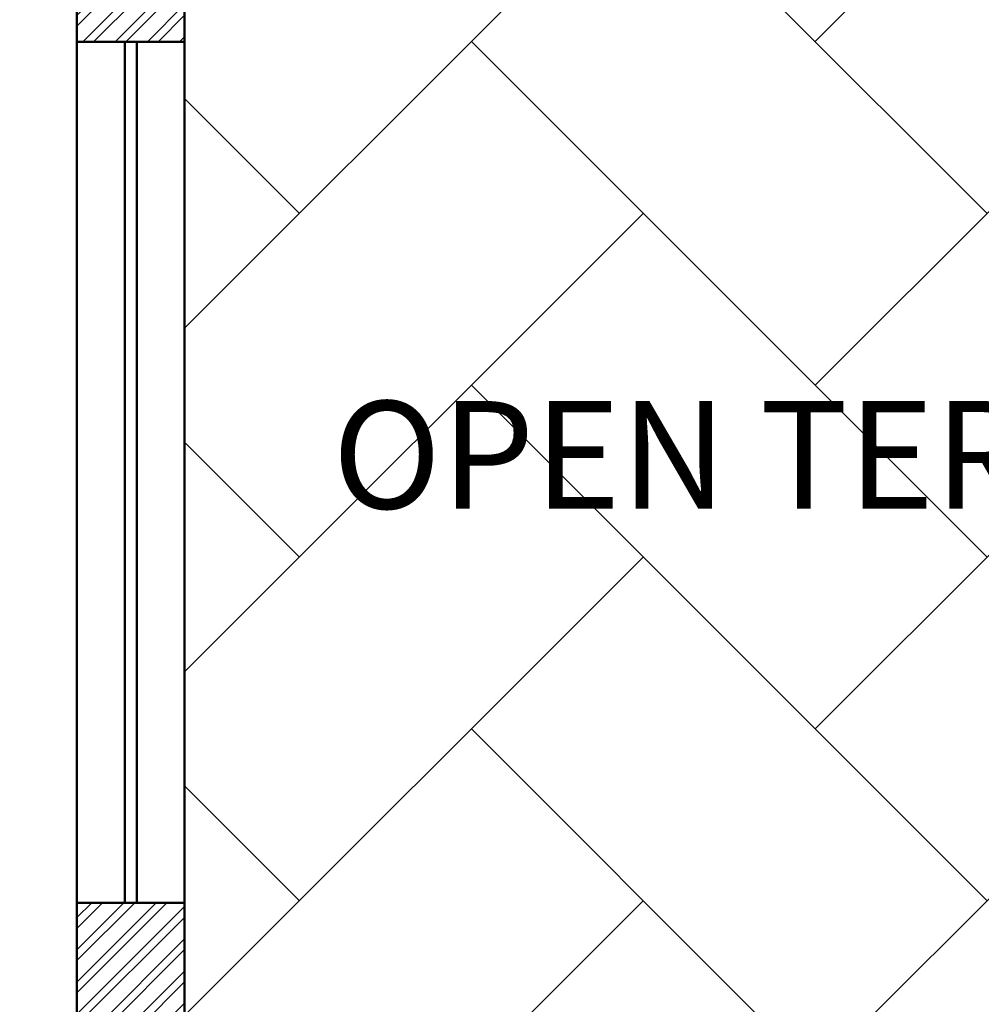
# Model space of a CAD drawing. Units: inches. Extents: x 3590 to 5167, y 65 to 1917.
# Tile 58 of 100: x 4919 to 5000, y 1558 to 1640. Entities that reach past the tile are written whole.
import ezdxf

# ---------------------------------------------------------------- set-up
doc = ezdxf.new("R2010")
doc.units = ezdxf.units.IN
for name, color, linetype, lineweight in [('A-AREA-IDEN', 7, 'Continuous', 18), ('A-FLOR-PATT', 8, 'Continuous', 13), ('A-WALL', 7, 'Continuous', 50), ('A-WALL-PATT', 251, 'Continuous', 13)]:
    doc.layers.add(name, color=color, linetype=linetype, lineweight=lineweight)
doc.styles.get("Standard").update_dxf_attribs({"font": 'arial.ttf'})

msp = doc.modelspace()

# ---------------------------------------------------------------- hatches: boundary and pattern name
at = {"layer": 'A-FLOR-PATT', "transparency": 33554687}
h = msp.add_hatch(dxfattribs=at)
h.set_pattern_fill('AR-HBONE', color=256, scale=0.2)
h.set_pattern_definition([(45, (-588.972, 0), (0, 28.73682), [60.96, -20.32]), (135, (-574.604, 14.368), (3e-15, 28.73682), [60.96, -20.32])])
h.paths.add_polyline_path([(5071.274, 1796.999), (4933.274, 1796.999), (4933.274, 1753.999), (4962.774, 1753.999, -0.414214), (4928.774, 1719.999), (4933.274, 1718.999), (4933.274, 1334.999), (5071.274, 1334.999)])
h.paths.add_polyline_path([(4951.78, 1521.077), (4951.715, 1521.04), (4951.563, 1520.895)], flags=16)
h.paths.add_polyline_path([(4952.267, 1521.376), (4952.198, 1521.371), (4952.198, 1521.356)], flags=0)
h.paths.add_polyline_path([(4967.051, 1529.728), (4965.231, 1528.694), (4963.411, 1527.714), (4961.756, 1526.851), (4963.589, 1527.449), (4964.036, 1527.478), (4962.975, 1527.249), (4961.76, 1526.852), (4959.792, 1525.834), (4958.005, 1524.895), (4956.24, 1523.93), (4954.504, 1522.919), (4954.129, 1522.682), (4953.361, 1521.997), (4953.366, 1521.998), (4953.605, 1522.064), (4955.106, 1522.761), (4956.921, 1523.434), (4958.678, 1523.915), (4960.358, 1524.2), (4961.945, 1524.286), (4964.171, 1524.108), (4965.958, 1523.309), (4963.863, 1522.976), (4965.187, 1522.499), (4963.366, 1522.497), (4961.545, 1522.487), (4959.764, 1522.461), (4958.304, 1522.419), (4957.974, 1522.388), (4956.307, 1522.232), (4954.718, 1522.071), (4953.251, 1521.899), (4953.525, 1521.623), (4954.331, 1521.379), (4956.243, 1521.23), (4958.039, 1520.93), (4959.684, 1520.483), (4961.16, 1519.896), (4963.107, 1518.8), (4964.393, 1517.325), (4962.973, 1517.726), (4964.558, 1516.661), (4965.407, 1515.708), (4963.507, 1516.322), (4961.68, 1517.005), (4959.935, 1517.745), (4958.282, 1518.528), (4956.732, 1519.343), (4955.295, 1520.175), (4954.672, 1520.572), (4954.513, 1520.627), (4955.658, 1519.318), (4956.703, 1517.982), (4957.644, 1516.647), (4958.485, 1515.334), (4959.55, 1513.524), (4960.438, 1511.769), (4958.841, 1513.62), (4957.452, 1515.325), (4955.819, 1517.459), (4956.665, 1515.448), (4957.111, 1513.923), (4957.447, 1511.714), (4957.076, 1509.793), (4956.538, 1511.11), (4955.992, 1512.569), (4955.444, 1514.125), (4954.898, 1515.735), (4954.357, 1517.356), (4953.824, 1518.943), (4953.305, 1520.452), (4953.065, 1521.116), (4952.971, 1521.146), (4952.949, 1521.086), (4952.73, 1520.199), (4953.37, 1518.024), (4953.757, 1516.373), (4954.051, 1514.765), (4954.264, 1513.221), (4954.471, 1511.131), (4954.497, 1510.402), (4954.409, 1511.76), (4954.264, 1513.221), (4954.051, 1514.765), (4953.757, 1516.373), (4953.37, 1518.024), (4952.877, 1519.698), (4952.716, 1520.141), (4952.533, 1519.059), (4952.374, 1517.789), (4952.219, 1516.312), (4952.046, 1514.6), (4951.833, 1512.626), (4951.557, 1510.363), (4951.203, 1512.168), (4950.852, 1514.339), (4950.985, 1516.376), (4951.66, 1518.286), (4952.593, 1520.481), (4952.357, 1521.13), (4951.855, 1520.328), (4950.839, 1518.908), (4949.777, 1517.587), (4948.916, 1516.617), (4948.111, 1515.256), (4947.089, 1513.554), (4945.889, 1511.615), (4946.326, 1513.402), (4946.562, 1514.249), (4945.528, 1513.327), (4944.581, 1512.531), (4946.018, 1514.508), (4947.204, 1516.048), (4947.893, 1517.313), (4949.307, 1518.764), (4950.414, 1519.767), (4950.451, 1519.806), (4952.267, 1521.376), (4951.645, 1521.493), (4950.404, 1521.18), (4948.044, 1520.359), (4946.119, 1519.452), (4944.572, 1518.475), (4943.35, 1517.443), (4941.997, 1515.92), (4941.661, 1515.275), (4942.813, 1516.99), (4944.572, 1518.475), (4946.119, 1519.452), (4948.044, 1520.359), (4950.404, 1521.18), (4951.645, 1521.493), (4949.647, 1521.868), (4948.6, 1521.756), (4947.126, 1521.57), (4945.42, 1521.348), (4943.45, 1521.105), (4941.183, 1520.856), (4942.86, 1521.613), (4943.873, 1522.03), (4942.952, 1521.909), (4941.41, 1521.485), (4939.543, 1520.67), (4938.968, 1520.226), (4940.733, 1521.299), (4942.952, 1521.909), (4943.702, 1522.008), (4945.894, 1522.7), (4947.565, 1522.714), (4948.921, 1522.566), (4951.131, 1522.183), (4950.971, 1522.297), (4948.129, 1523.006), (4946.035, 1523.707), (4944.232, 1524.521), (4942.707, 1525.461), (4941.444, 1526.537), (4940.43, 1527.761), (4939.649, 1529.143), (4941.421, 1528.122), (4943.147, 1527.132), (4944.841, 1526.175), (4946.514, 1525.25), (4948.179, 1524.359), (4948.365, 1524.263), (4946.475, 1526.045), (4945.181, 1527.54), (4944.19, 1529.033), (4943.496, 1530.54), (4943.278, 1531.36), (4942.498, 1531.919), (4943.114, 1531.762), (4942.959, 1533.659), (4944.14, 1531.989), (4944.612, 1531.323), (4946.202, 1530.463), (4947.486, 1529.509), (4948.79, 1528.226), (4950.368, 1526.237), (4949.485, 1528.155), (4948.851, 1530.123), (4948.491, 1532.041), (4948.381, 1533.918), (4948.501, 1535.76), (4948.827, 1537.573), (4949.418, 1535.565), (4949.957, 1533.569), (4950.464, 1531.586), (4950.961, 1529.617), (4951.391, 1527.954), (4951.724, 1530.687), (4952.201, 1532.58), (4952.889, 1534.33), (4953.77, 1535.951), (4954.827, 1537.46), (4954.521, 1535.39), (4954.273, 1533.937), (4955.58, 1535.663), (4956.748, 1536.739), (4956.159, 1534.78), (4955.589, 1532.873), (4955.043, 1531.006), (4954.525, 1529.166), (4954.038, 1527.341), (4953.638, 1525.733), (4953.611, 1525.586), (4953.398, 1524.166), (4953.382, 1524.009), (4954.07, 1525.476), (4954.912, 1527.022), (4956.136, 1528.894), (4957.847, 1530.577), (4959.376, 1531.54), (4958.256, 1530.104), (4957.143, 1528.663), (4956.066, 1527.243), (4955.056, 1525.871), (4954.141, 1524.571), (4953.352, 1523.372), (4953.311, 1523.303), (4953.273, 1522.925), (4953.261, 1522.382), (4954.103, 1523.373), (4954.63, 1524.284), (4955.961, 1526.358), (4957.23, 1528.13), (4958.421, 1529.609), (4960.037, 1531.368), (4961.374, 1532.375), (4962.101, 1532.77), (4961.07, 1531.061), (4959.987, 1529.438), (4958.869, 1527.908), (4958.15, 1527.007), (4959.803, 1528.003), (4961.589, 1528.793), (4963.391, 1529.328), (4965.211, 1529.632)], flags=16)
h.paths.add_polyline_path([(4962.944, 1523.182), (4961.107, 1523.422), (4960.392, 1523.362), (4962.35, 1523.331)], flags=0)
h.paths.add_polyline_path([(5049.541, 1584.551), (5049.476, 1584.515), (5049.325, 1584.37)], flags=16)
h.paths.add_polyline_path([(5050.028, 1584.851), (5049.959, 1584.845), (5049.959, 1584.83)], flags=0)
h.paths.add_polyline_path([(5042.333, 1581.949), (5043.88, 1582.926), (5045.806, 1583.833), (5048.165, 1584.654), (5049.406, 1584.967), (5047.408, 1585.342), (5046.361, 1585.231), (5044.888, 1585.044), (5043.181, 1584.822), (5041.211, 1584.579), (5038.944, 1584.33), (5040.622, 1585.087), (5041.634, 1585.504), (5040.713, 1585.383), (5039.171, 1584.959), (5037.304, 1584.144), (5036.729, 1583.7), (5038.494, 1584.773), (5040.713, 1585.383), (5041.463, 1585.482), (5043.655, 1586.174), (5045.326, 1586.188), (5046.682, 1586.04), (5048.893, 1585.657), (5048.732, 1585.771), (5045.891, 1586.48), (5043.796, 1587.181), (5041.994, 1587.996), (5040.468, 1588.935), (5039.205, 1590.011), (5038.191, 1591.235), (5037.41, 1592.617), (5039.182, 1591.596), (5040.909, 1590.607), (5042.602, 1589.649), (5044.275, 1588.724), (5045.94, 1587.833), (5046.126, 1587.738), (5044.237, 1589.519), (5042.942, 1591.015), (5041.952, 1592.508), (5041.257, 1594.014), (5041.039, 1594.834), (5040.26, 1595.393), (5040.875, 1595.237), (5040.721, 1597.133), (5041.901, 1595.463), (5042.373, 1594.798), (5043.963, 1593.938), (5045.247, 1592.983), (5046.552, 1591.701), (5048.129, 1589.712), (5047.247, 1591.63), (5046.613, 1593.597), (5046.252, 1595.515), (5046.142, 1597.392), (5046.262, 1599.234), (5046.588, 1601.047), (5047.179, 1599.039), (5047.718, 1597.043), (5048.225, 1595.06), (5048.722, 1593.091), (5049.152, 1591.429), (5049.485, 1594.161), (5049.962, 1596.054), (5050.65, 1597.804), (5051.532, 1599.425), (5052.589, 1600.934), (5052.283, 1598.864), (5052.034, 1597.411), (5053.341, 1599.137), (5054.509, 1600.213), (5053.92, 1598.254), (5053.35, 1596.348), (5052.805, 1594.48), (5052.286, 1592.64), (5051.799, 1590.815), (5051.4, 1589.207), (5051.373, 1589.06), (5051.159, 1587.64), (5051.143, 1587.483), (5051.831, 1588.95), (5052.673, 1590.496), (5053.898, 1592.368), (5055.608, 1594.051), (5057.137, 1595.014), (5056.017, 1593.578), (5054.904, 1592.137), (5053.828, 1590.717), (5052.817, 1589.345), (5051.902, 1588.046), (5051.113, 1586.846), (5051.072, 1586.777), (5051.034, 1586.399), (5051.022, 1585.856), (5051.864, 1586.847), (5052.391, 1587.758), (5053.723, 1589.832), (5054.991, 1591.604), (5056.182, 1593.083), (5057.798, 1594.842), (5059.135, 1595.849), (5059.863, 1596.244), (5058.831, 1594.535), (5057.749, 1592.912), (5056.63, 1591.382), (5055.912, 1590.482), (5057.564, 1591.477), (5059.35, 1592.267), (5061.152, 1592.802), (5062.972, 1593.106), (5064.812, 1593.203), (5062.992, 1592.169), (5061.172, 1591.188), (5059.518, 1590.325), (5061.35, 1590.924), (5061.797, 1590.952), (5060.737, 1590.723), (5059.521, 1590.326), (5057.553, 1589.308), (5055.766, 1588.369), (5054.002, 1587.404), (5052.265, 1586.393), (5051.891, 1586.156), (5051.122, 1585.471), (5051.127, 1585.472), (5051.366, 1585.538), (5052.867, 1586.235), (5054.682, 1586.908), (5056.439, 1587.389), (5058.12, 1587.675), (5059.706, 1587.76), (5061.933, 1587.583), (5063.719, 1586.783), (5061.624, 1586.45), (5062.949, 1585.973), (5061.127, 1585.971), (5059.307, 1585.961), (5057.525, 1585.935), (5056.065, 1585.893), (5055.735, 1585.862), (5054.068, 1585.707), (5052.479, 1585.546), (5051.012, 1585.373), (5051.286, 1585.097), (5052.092, 1584.853), (5054.004, 1584.704), (5055.8, 1584.404), (5057.446, 1583.958), (5058.921, 1583.37), (5060.868, 1582.274), (5062.154, 1580.799), (5060.734, 1581.2), (5062.32, 1580.135), (5063.168, 1579.182), (5061.269, 1579.796), (5059.441, 1580.479), (5057.696, 1581.219), (5056.043, 1582.003), (5054.493, 1582.817), (5053.057, 1583.649), (5052.433, 1584.047), (5052.274, 1584.101), (5053.42, 1582.793), (5054.464, 1581.457), (5055.405, 1580.121), (5056.247, 1578.809), (5057.311, 1576.998), (5058.199, 1575.244), (5056.602, 1577.094), (5055.213, 1578.799), (5053.58, 1580.933), (5054.427, 1578.922), (5054.872, 1577.397), (5055.208, 1575.189), (5054.838, 1573.267), (5054.299, 1574.584), (5053.754, 1576.043), (5053.206, 1577.599), (5052.659, 1579.209), (5052.118, 1580.83), (5051.585, 1582.417), (5051.066, 1583.927), (5050.826, 1584.59), (5050.733, 1584.62), (5050.711, 1584.561), (5050.491, 1583.673), (5051.131, 1581.498), (5051.518, 1579.847), (5051.813, 1578.24), (5052.026, 1576.695), (5052.233, 1574.605), (5052.258, 1573.876), (5052.17, 1575.234), (5052.026, 1576.695), (5051.813, 1578.24), (5051.518, 1579.847), (5051.131, 1581.498), (5050.638, 1583.172), (5050.477, 1583.615), (5050.294, 1582.533), (5050.136, 1581.263), (5049.981, 1579.786), (5049.807, 1578.074), (5049.594, 1576.1), (5049.318, 1573.837), (5048.965, 1575.642), (5048.613, 1577.813), (5048.747, 1579.85), (5049.421, 1581.76), (5050.354, 1583.955), (5050.118, 1584.604), (5049.616, 1583.802), (5048.6, 1582.382), (5047.538, 1581.061), (5046.677, 1580.091), (5045.872, 1578.73), (5044.85, 1577.028), (5043.651, 1575.089), (5044.087, 1576.877), (5044.324, 1577.723), (5043.289, 1576.801), (5042.342, 1576.005), (5043.779, 1577.982), (5044.966, 1579.522), (5045.655, 1580.787), (5047.068, 1582.239), (5048.175, 1583.241), (5048.213, 1583.28), (5050.028, 1584.851), (5049.406, 1584.967), (5048.165, 1584.654), (5045.806, 1583.833), (5043.88, 1582.926), (5042.333, 1581.949), (5041.111, 1580.917), (5039.758, 1579.394), (5039.423, 1578.749), (5040.575, 1580.464)], flags=16)
h.paths.add_polyline_path([(4954.799, 1533.12), (4954.262, 1532.079), (4953.831, 1530.935), (4953.505, 1529.636), (4953.283, 1528.133), (4953.167, 1526.376), (4953.156, 1524.315), (4953.277, 1521.236), (4952.802, 1521.842), (4951.557, 1521.998), (4950.976, 1521.961), (4952.661, 1521.941), (4952.802, 1521.842), (4953.152, 1523.593), (4953.167, 1526.376), (4953.283, 1528.133), (4953.609, 1530.346), (4954.456, 1532.592)], flags=0)
h.paths.add_polyline_path([(5050.563, 1585.316), (5049.318, 1585.472), (5048.737, 1585.435), (5050.422, 1585.415), (5050.563, 1585.316), (5050.914, 1587.067), (5050.928, 1589.851), (5051.045, 1591.607), (5051.371, 1593.82), (5052.217, 1596.066), (5052.56, 1596.594), (5052.024, 1595.554), (5051.592, 1594.409), (5051.266, 1593.11), (5051.045, 1591.607), (5050.928, 1589.851), (5050.918, 1587.789), (5051.038, 1584.71)], flags=0)
h.paths.add_polyline_path([(5058.153, 1586.836), (5060.111, 1586.805), (5060.705, 1586.656), (5058.868, 1586.896)], flags=0)
h.paths.add_polyline_path([(5049.541, 1430.936), (5049.476, 1430.9), (5049.325, 1430.755)], flags=16)
h.paths.add_polyline_path([(5050.028, 1431.236), (5049.959, 1431.231), (5049.959, 1431.215)], flags=0)
h.paths.add_polyline_path([(5046.588, 1447.432), (5047.179, 1445.425), (5047.718, 1443.429), (5048.225, 1441.446), (5048.722, 1439.476), (5049.152, 1437.814), (5049.485, 1440.546), (5049.962, 1442.439), (5050.65, 1444.189), (5051.532, 1445.811), (5052.589, 1447.319), (5052.283, 1445.249), (5052.034, 1443.796), (5053.341, 1445.522), (5054.509, 1446.598), (5053.92, 1444.64), (5053.35, 1442.733), (5052.805, 1440.865), (5052.286, 1439.025), (5051.799, 1437.201), (5051.4, 1435.592), (5051.373, 1435.445), (5051.159, 1434.025), (5051.143, 1433.868), (5051.831, 1435.335), (5052.673, 1436.881), (5053.898, 1438.753), (5055.608, 1440.436), (5057.137, 1441.4), (5056.017, 1439.963), (5054.904, 1438.522), (5053.828, 1437.102), (5052.817, 1435.73), (5051.902, 1434.431), (5051.113, 1433.231), (5051.072, 1433.162), (5051.034, 1432.784), (5051.022, 1432.242), (5051.864, 1433.232), (5052.391, 1434.143), (5053.723, 1436.217), (5054.991, 1437.989), (5056.182, 1439.468), (5057.798, 1441.227), (5059.135, 1442.235), (5059.863, 1442.629), (5058.831, 1440.921), (5057.749, 1439.298), (5056.63, 1437.767), (5055.912, 1436.867), (5057.564, 1437.863), (5059.35, 1438.652), (5061.152, 1439.187), (5062.972, 1439.491), (5064.812, 1439.588), (5062.992, 1438.554), (5061.172, 1437.573), (5059.518, 1436.71), (5061.35, 1437.309), (5061.797, 1437.337), (5060.737, 1437.108), (5059.521, 1436.711), (5057.553, 1435.693), (5055.766, 1434.754), (5054.002, 1433.789), (5052.265, 1432.778), (5051.891, 1432.541), (5051.122, 1431.856), (5051.127, 1431.857), (5051.366, 1431.923), (5052.867, 1432.62), (5054.682, 1433.293), (5056.439, 1433.775), (5058.12, 1434.06), (5059.706, 1434.145), (5061.933, 1433.968), (5063.719, 1433.168), (5061.624, 1432.835), (5062.949, 1432.358), (5061.127, 1432.357), (5059.307, 1432.346), (5057.525, 1432.32), (5056.065, 1432.278), (5055.735, 1432.248), (5054.068, 1432.092), (5052.479, 1431.931), (5051.012, 1431.759), (5051.286, 1431.482), (5052.092, 1431.238), (5054.004, 1431.089), (5055.8, 1430.789), (5057.446, 1430.343), (5058.921, 1429.755), (5060.868, 1428.66), (5062.154, 1427.185), (5060.734, 1427.585), (5062.32, 1426.52), (5063.168, 1425.567), (5061.269, 1426.181), (5059.441, 1426.865), (5057.696, 1427.604), (5056.043, 1428.388), (5054.493, 1429.202), (5053.057, 1430.034), (5052.433, 1430.432), (5052.274, 1430.487), (5053.42, 1429.178), (5054.464, 1427.842), (5055.405, 1426.506), (5056.247, 1425.194), (5057.311, 1423.383), (5058.199, 1421.629), (5056.602, 1423.479), (5055.213, 1425.184), (5053.58, 1427.318), (5054.427, 1425.307), (5054.872, 1423.782), (5055.208, 1421.574), (5054.838, 1419.652), (5054.299, 1420.97), (5053.754, 1422.428), (5053.206, 1423.984), (5052.659, 1425.595), (5052.118, 1427.215), (5051.585, 1428.802), (5051.066, 1430.312), (5050.826, 1430.975), (5050.733, 1431.005), (5050.711, 1430.946), (5050.491, 1430.058), (5051.131, 1427.883), (5051.518, 1426.232), (5051.813, 1424.625), (5052.026, 1423.081), (5052.233, 1420.991), (5052.258, 1420.261), (5052.17, 1421.619), (5052.026, 1423.081), (5051.813, 1424.625), (5051.518, 1426.232), (5051.131, 1427.883), (5050.638, 1429.558), (5050.477, 1430.001), (5050.294, 1428.918), (5050.136, 1427.648), (5049.981, 1426.171), (5049.807, 1424.459), (5049.594, 1422.485), (5049.318, 1420.222), (5048.965, 1422.028), (5048.613, 1424.199), (5048.747, 1426.235), (5049.421, 1428.146), (5050.354, 1430.34), (5050.118, 1430.989), (5049.616, 1430.187), (5048.6, 1428.768), (5047.538, 1427.446), (5046.677, 1426.477), (5045.872, 1425.116), (5044.85, 1423.413), (5043.651, 1421.474), (5044.087, 1423.262), (5044.324, 1424.109), (5043.289, 1423.186), (5042.342, 1422.391), (5043.779, 1424.368), (5044.966, 1425.907), (5045.655, 1427.173), (5047.068, 1428.624), (5048.175, 1429.627), (5048.213, 1429.666), (5050.028, 1431.236), (5049.406, 1431.353), (5048.165, 1431.039), (5045.806, 1430.218), (5043.88, 1429.311), (5042.333, 1428.334), (5041.111, 1427.302), (5039.758, 1425.779), (5039.423, 1425.134), (5040.575, 1426.849), (5042.333, 1428.334), (5043.88, 1429.311), (5045.806, 1430.218), (5048.165, 1431.039), (5049.406, 1431.353), (5047.408, 1431.727), (5046.361, 1431.616), (5044.888, 1431.429), (5043.181, 1431.207), (5041.211, 1430.964), (5038.944, 1430.715), (5040.622, 1431.472), (5041.634, 1431.89), (5040.713, 1431.769), (5039.171, 1431.345), (5037.304, 1430.53), (5036.729, 1430.085), (5038.494, 1431.158), (5040.713, 1431.769), (5041.463, 1431.867), (5043.655, 1432.559), (5045.326, 1432.573), (5046.682, 1432.425), (5048.893, 1432.042), (5048.732, 1432.156), (5045.891, 1432.865), (5043.796, 1433.566), (5041.994, 1434.381), (5040.468, 1435.321), (5039.205, 1436.396), (5038.191, 1437.62), (5037.41, 1439.002), (5039.182, 1437.982), (5040.909, 1436.992), (5042.602, 1436.034), (5044.275, 1435.109), (5045.94, 1434.218), (5046.126, 1434.123), (5044.237, 1435.904), (5042.942, 1437.4), (5041.952, 1438.893), (5041.257, 1440.399), (5041.039, 1441.219), (5040.26, 1441.778), (5040.875, 1441.622), (5040.721, 1443.518), (5041.901, 1441.848), (5042.373, 1441.183), (5043.963, 1440.323), (5045.247, 1439.369), (5046.552, 1438.086), (5048.129, 1436.097), (5047.247, 1438.015), (5046.613, 1439.982), (5046.252, 1441.901), (5046.142, 1443.778), (5046.262, 1445.619)], flags=16)
h.paths.add_polyline_path([(5052.382, 1444.255), (5051.623, 1442.78), (5052.024, 1441.939), (5052.56, 1442.98)], flags=0)
h.paths.add_polyline_path([(5050.563, 1431.701), (5049.318, 1431.857), (5048.737, 1431.821), (5050.422, 1431.8)], flags=0)
h.paths.add_polyline_path([(5058.153, 1433.221), (5060.111, 1433.19), (5060.705, 1433.041), (5058.868, 1433.281)], flags=0)
h.paths.add_polyline_path([(5049.541, 1352.285), (5049.476, 1352.249), (5049.325, 1352.104)], flags=16)
h.paths.add_polyline_path([(5050.028, 1352.585), (5049.959, 1352.58), (5049.959, 1352.564)], flags=0)
h.paths.add_polyline_path([(5046.588, 1368.781), (5047.179, 1366.774), (5047.718, 1364.778), (5048.225, 1362.795), (5048.722, 1360.825), (5049.152, 1359.163), (5049.485, 1361.896), (5049.962, 1363.789), (5050.65, 1365.538), (5051.532, 1367.16), (5052.589, 1368.669), (5052.283, 1366.598), (5052.034, 1365.145), (5053.341, 1366.871), (5054.509, 1367.947), (5053.92, 1365.989), (5053.35, 1364.082), (5052.805, 1362.214), (5052.286, 1360.374), (5051.799, 1358.55), (5051.4, 1356.942), (5051.373, 1356.794), (5051.159, 1355.374), (5051.143, 1355.218), (5051.831, 1356.684), (5052.673, 1358.23), (5053.898, 1360.102), (5055.608, 1361.786), (5057.137, 1362.749), (5056.017, 1361.313), (5054.904, 1359.872), (5053.828, 1358.452), (5052.817, 1357.079), (5051.902, 1355.78), (5051.113, 1354.581), (5051.072, 1354.512), (5051.034, 1354.133), (5051.022, 1353.591), (5051.864, 1354.581), (5052.391, 1355.492), (5053.723, 1357.566), (5054.991, 1359.338), (5056.182, 1360.817), (5057.798, 1362.577), (5059.135, 1363.584), (5059.863, 1363.979), (5058.831, 1362.27), (5057.749, 1360.647), (5056.63, 1359.117), (5055.912, 1358.216), (5057.564, 1359.212), (5059.35, 1360.001), (5061.152, 1360.536), (5062.972, 1360.841), (5064.812, 1360.937), (5062.992, 1359.903), (5061.172, 1358.923), (5059.518, 1358.059), (5061.35, 1358.658), (5061.797, 1358.687), (5060.737, 1358.458), (5059.521, 1358.061), (5057.553, 1357.043), (5055.766, 1356.103), (5054.002, 1355.138), (5052.265, 1354.127), (5051.891, 1353.89), (5051.122, 1353.206), (5051.127, 1353.206), (5051.366, 1353.272), (5052.867, 1353.969), (5054.682, 1354.643), (5056.439, 1355.124), (5058.12, 1355.409), (5059.706, 1355.495), (5061.933, 1355.317), (5063.719, 1354.518), (5061.624, 1354.184), (5062.949, 1353.708), (5061.127, 1353.706), (5059.307, 1353.695), (5057.525, 1353.669), (5056.065, 1353.627), (5055.735, 1353.597), (5054.068, 1353.441), (5052.479, 1353.28), (5051.012, 1353.108), (5051.286, 1352.831), (5052.092, 1352.587), (5054.004, 1352.439), (5055.8, 1352.138), (5057.446, 1351.692), (5058.921, 1351.104), (5060.868, 1350.009), (5062.154, 1348.534), (5060.734, 1348.935), (5062.32, 1347.869), (5063.168, 1346.916), (5061.269, 1347.53), (5059.441, 1348.214), (5057.696, 1348.954), (5056.043, 1349.737), (5054.493, 1350.551), (5053.057, 1351.383), (5052.433, 1351.781), (5052.274, 1351.836), (5053.42, 1350.527), (5054.464, 1349.191), (5055.405, 1347.855), (5056.247, 1346.543), (5057.311, 1344.733), (5058.199, 1342.978), (5056.602, 1344.828), (5055.213, 1346.534), (5053.58, 1348.667), (5054.427, 1346.656), (5054.872, 1345.132), (5055.208, 1342.923), (5054.838, 1341.002), (5054.299, 1342.319), (5053.754, 1343.778), (5053.206, 1345.334), (5052.659, 1346.944), (5052.118, 1348.564), (5051.585, 1350.151), (5051.066, 1351.661), (5050.826, 1352.324), (5050.733, 1352.355), (5050.711, 1352.295), (5050.491, 1351.408), (5051.131, 1349.232), (5051.518, 1347.581), (5051.813, 1345.974), (5052.026, 1344.43), (5052.233, 1342.34), (5052.258, 1341.61), (5052.17, 1342.969), (5052.026, 1344.43), (5051.813, 1345.974), (5051.518, 1347.581), (5051.131, 1349.232), (5050.638, 1350.907), (5050.477, 1351.35), (5050.294, 1350.267), (5050.136, 1348.997), (5049.981, 1347.52), (5049.807, 1345.809), (5049.594, 1343.835), (5049.318, 1341.571), (5048.965, 1343.377), (5048.613, 1345.548), (5048.747, 1347.585), (5049.421, 1349.495), (5050.354, 1351.689), (5050.118, 1352.339), (5049.616, 1351.536), (5048.6, 1350.117), (5047.538, 1348.795), (5046.677, 1347.826), (5045.872, 1346.465), (5044.85, 1344.763), (5043.651, 1342.824), (5044.087, 1344.611), (5044.324, 1345.458), (5043.289, 1344.535), (5042.342, 1343.74), (5043.779, 1345.717), (5044.966, 1347.256), (5045.655, 1348.522), (5047.068, 1349.973), (5048.175, 1350.976), (5048.213, 1351.015), (5050.028, 1352.585), (5049.406, 1352.702), (5048.165, 1352.388), (5045.806, 1351.567), (5043.88, 1350.661), (5042.333, 1349.683), (5041.111, 1348.651), (5039.758, 1347.128), (5039.423, 1346.483), (5040.575, 1348.198), (5042.333, 1349.683), (5043.88, 1350.661), (5045.806, 1351.567), (5048.165, 1352.388), (5049.406, 1352.702), (5047.408, 1353.076), (5046.361, 1352.965), (5044.888, 1352.779), (5043.181, 1352.556), (5041.211, 1352.313), (5038.944, 1352.065), (5040.622, 1352.821), (5041.634, 1353.239), (5040.713, 1353.118), (5039.171, 1352.694), (5037.304, 1351.879), (5036.729, 1351.434), (5038.494, 1352.508), (5040.713, 1353.118), (5041.463, 1353.216), (5043.655, 1353.909), (5045.326, 1353.923), (5046.682, 1353.774), (5048.893, 1353.391), (5048.732, 1353.506), (5045.891, 1354.214), (5043.796, 1354.915), (5041.994, 1355.73), (5040.468, 1356.67), (5039.205, 1357.746), (5038.191, 1358.969), (5037.41, 1360.352), (5039.182, 1359.331), (5040.909, 1358.341), (5042.602, 1357.383), (5044.275, 1356.458), (5045.94, 1355.567), (5046.126, 1355.472), (5044.237, 1357.253), (5042.942, 1358.749), (5041.952, 1360.242), (5041.257, 1361.748), (5041.039, 1362.568), (5040.26, 1363.128), (5040.875, 1362.971), (5040.721, 1364.867), (5041.901, 1363.197), (5042.373, 1362.532), (5043.963, 1361.672), (5045.247, 1360.718), (5046.552, 1359.435), (5048.129, 1357.446), (5047.247, 1359.364), (5046.613, 1361.331), (5046.252, 1363.25), (5046.142, 1365.127), (5046.262, 1366.969)], flags=16)
h.paths.add_polyline_path([(5052.382, 1365.604), (5051.623, 1364.129), (5052.024, 1363.288), (5052.56, 1364.329)], flags=0)
h.paths.add_polyline_path([(4951.78, 1698.041), (4951.715, 1698.005), (4951.563, 1697.859)], flags=16)
h.paths.add_polyline_path([(4952.267, 1698.341), (4952.198, 1698.335), (4952.198, 1698.32)], flags=0)
h.paths.add_polyline_path([(4957.076, 1686.757), (4956.538, 1688.074), (4955.992, 1689.533), (4955.444, 1691.089), (4954.898, 1692.699), (4954.357, 1694.32), (4953.824, 1695.907), (4953.305, 1697.417), (4953.065, 1698.08), (4952.971, 1698.11), (4952.949, 1698.051), (4952.73, 1697.163), (4953.37, 1694.988), (4953.757, 1693.337), (4954.051, 1691.729), (4954.264, 1690.185), (4954.471, 1688.095), (4954.497, 1687.366), (4954.409, 1688.724), (4954.264, 1690.185), (4954.051, 1691.729), (4953.757, 1693.337), (4953.37, 1694.988), (4952.877, 1696.662), (4952.716, 1697.105), (4952.533, 1696.023), (4952.374, 1694.753), (4952.219, 1693.276), (4952.046, 1691.564), (4951.833, 1689.59), (4951.557, 1687.327), (4951.203, 1689.132), (4950.852, 1691.303), (4950.985, 1693.34), (4951.66, 1695.25), (4952.593, 1697.445), (4952.357, 1698.094), (4951.855, 1697.292), (4950.839, 1695.872), (4949.777, 1694.551), (4948.916, 1693.581), (4948.111, 1692.22), (4947.089, 1690.518), (4945.889, 1688.579), (4946.326, 1690.366), (4946.562, 1691.213), (4945.528, 1690.291), (4944.581, 1689.495), (4946.018, 1691.472), (4947.204, 1693.012), (4947.893, 1694.277), (4949.307, 1695.729), (4950.414, 1696.731), (4950.451, 1696.77), (4952.267, 1698.341), (4951.645, 1698.457), (4950.404, 1698.144), (4948.044, 1697.323), (4946.119, 1696.416), (4944.572, 1695.439), (4943.35, 1694.407), (4941.997, 1692.884), (4941.661, 1692.239), (4942.813, 1693.954), (4944.572, 1695.439), (4946.119, 1696.416), (4948.044, 1697.323), (4950.404, 1698.144), (4951.645, 1698.457), (4949.647, 1698.832), (4948.6, 1698.72), (4947.126, 1698.534), (4945.42, 1698.312), (4943.45, 1698.069), (4941.183, 1697.82), (4942.86, 1698.577), (4943.873, 1698.994), (4942.952, 1698.873), (4941.41, 1698.449), (4939.543, 1697.634), (4938.968, 1697.19), (4940.733, 1698.263), (4942.952, 1698.873), (4943.702, 1698.972), (4945.894, 1699.664), (4947.565, 1699.678), (4948.921, 1699.53), (4951.131, 1699.147), (4950.971, 1699.261), (4948.129, 1699.97), (4946.035, 1700.671), (4944.232, 1701.486), (4942.707, 1702.425), (4941.444, 1703.501), (4940.43, 1704.725), (4939.649, 1706.107), (4941.421, 1705.086), (4943.147, 1704.097), (4944.841, 1703.139), (4946.514, 1702.214), (4948.179, 1701.323), (4948.365, 1701.227), (4946.475, 1703.009), (4945.181, 1704.505), (4944.19, 1705.997), (4943.496, 1707.504), (4943.278, 1708.324), (4942.498, 1708.883), (4943.114, 1708.727), (4942.959, 1710.623), (4944.14, 1708.953), (4944.612, 1708.287), (4946.202, 1707.428), (4947.486, 1706.473), (4948.79, 1705.191), (4950.368, 1703.202), (4949.485, 1705.12), (4948.851, 1707.087), (4948.491, 1709.005), (4948.381, 1710.882), (4948.501, 1712.724), (4948.827, 1714.537), (4949.418, 1712.529), (4949.957, 1710.533), (4950.464, 1708.55), (4950.961, 1706.581), (4951.391, 1704.919), (4951.724, 1707.651), (4952.201, 1709.544), (4952.889, 1711.294), (4953.77, 1712.915), (4954.827, 1714.424), (4954.521, 1712.354), (4954.273, 1710.901), (4955.58, 1712.627), (4956.748, 1713.703), (4956.159, 1711.744), (4955.589, 1709.837), (4955.043, 1707.97), (4954.525, 1706.13), (4954.038, 1704.305), (4953.638, 1702.697), (4953.611, 1702.55), (4953.398, 1701.13), (4953.382, 1700.973), (4954.07, 1702.44), (4954.912, 1703.986), (4956.136, 1705.858), (4957.847, 1707.541), (4959.376, 1708.504), (4958.256, 1707.068), (4957.143, 1705.627), (4956.066, 1704.207), (4955.056, 1702.835), (4954.141, 1701.536), (4953.352, 1700.336), (4953.311, 1700.267), (4953.273, 1699.889), (4953.261, 1699.346), (4954.103, 1700.337), (4954.63, 1701.248), (4955.961, 1703.322), (4957.23, 1705.094), (4958.421, 1706.573), (4960.037, 1708.332), (4961.374, 1709.339), (4962.101, 1709.734), (4961.07, 1708.025), (4959.987, 1706.402), (4958.869, 1704.872), (4958.15, 1703.972), (4959.803, 1704.967), (4961.589, 1705.757), (4963.391, 1706.292), (4965.211, 1706.596), (4967.051, 1706.692), (4965.231, 1705.659), (4963.411, 1704.678), (4961.756, 1703.815), (4963.589, 1704.413), (4964.036, 1704.442), (4962.975, 1704.213), (4961.76, 1703.816), (4959.792, 1702.798), (4958.005, 1701.859), (4956.24, 1700.894), (4954.504, 1699.883), (4954.129, 1699.646), (4953.361, 1698.961), (4953.366, 1698.962), (4953.605, 1699.028), (4955.106, 1699.725), (4956.921, 1700.398), (4958.678, 1700.879), (4960.358, 1701.164), (4961.945, 1701.25), (4964.171, 1701.073), (4965.958, 1700.273), (4963.863, 1699.94), (4965.187, 1699.463), (4963.366, 1699.461), (4961.545, 1699.451), (4959.764, 1699.425), (4958.304, 1699.383), (4957.974, 1699.352), (4956.307, 1699.197), (4954.718, 1699.036), (4953.251, 1698.863), (4953.525, 1698.587), (4954.331, 1698.343), (4956.243, 1698.194), (4958.039, 1697.894), (4959.684, 1697.447), (4961.16, 1696.86), (4963.107, 1695.764), (4964.393, 1694.289), (4962.973, 1694.69), (4964.558, 1693.625), (4965.407, 1692.672), (4963.507, 1693.286), (4961.68, 1693.969), (4959.935, 1694.709), (4958.282, 1695.492), (4956.732, 1696.307), (4955.295, 1697.139), (4954.672, 1697.536), (4954.513, 1697.591), (4955.658, 1696.282), (4956.703, 1694.946), (4957.644, 1693.611), (4958.485, 1692.298), (4959.55, 1690.488), (4960.438, 1688.733), (4958.841, 1690.584), (4957.452, 1692.289), (4955.819, 1694.423), (4956.665, 1692.412), (4957.111, 1690.887), (4957.447, 1688.678)], flags=16)
h.paths.add_polyline_path([(5050.563, 1353.05), (5049.318, 1353.207), (5048.737, 1353.17), (5050.422, 1353.15)], flags=0)
h.paths.add_polyline_path([(4951.78, 1351.486), (4951.715, 1351.45), (4951.563, 1351.305)], flags=16)
h.paths.add_polyline_path([(4952.267, 1351.786), (4952.198, 1351.78), (4952.198, 1351.765)], flags=0)
h.paths.add_polyline_path([(4954.827, 1367.869), (4954.521, 1365.799), (4954.273, 1364.346), (4955.58, 1366.072), (4956.748, 1367.148), (4956.159, 1365.19), (4955.589, 1363.283), (4955.043, 1361.415), (4954.525, 1359.575), (4954.038, 1357.751), (4953.638, 1356.142), (4953.611, 1355.995), (4953.398, 1354.575), (4953.382, 1354.418), (4954.07, 1355.885), (4954.912, 1357.431), (4956.136, 1359.303), (4957.847, 1360.986), (4959.376, 1361.95), (4958.256, 1360.513), (4957.143, 1359.072), (4956.066, 1357.652), (4955.056, 1356.28), (4954.141, 1354.981), (4953.352, 1353.781), (4953.311, 1353.712), (4953.273, 1353.334), (4953.261, 1352.792), (4954.103, 1353.782), (4954.63, 1354.693), (4955.961, 1356.767), (4957.23, 1358.539), (4958.421, 1360.018), (4960.037, 1361.777), (4961.374, 1362.785), (4962.101, 1363.179), (4961.07, 1361.471), (4959.987, 1359.848), (4958.869, 1358.317), (4958.15, 1357.417), (4959.803, 1358.413), (4961.589, 1359.202), (4963.391, 1359.737), (4965.211, 1360.041), (4967.051, 1360.138), (4965.231, 1359.104), (4963.411, 1358.123), (4961.756, 1357.26), (4963.589, 1357.859), (4964.036, 1357.887), (4962.975, 1357.658), (4961.76, 1357.261), (4959.792, 1356.243), (4958.005, 1355.304), (4956.24, 1354.339), (4954.504, 1353.328), (4954.129, 1353.091), (4953.361, 1352.406), (4953.366, 1352.407), (4953.605, 1352.473), (4955.106, 1353.17), (4956.921, 1353.843), (4958.678, 1354.325), (4960.358, 1354.61), (4961.945, 1354.695), (4964.171, 1354.518), (4965.958, 1353.718), (4963.863, 1353.385), (4965.187, 1352.908), (4963.366, 1352.907), (4961.545, 1352.896), (4959.764, 1352.87), (4958.304, 1352.828), (4957.974, 1352.798), (4956.307, 1352.642), (4954.718, 1352.481), (4953.251, 1352.309), (4953.525, 1352.032), (4954.331, 1351.788), (4956.243, 1351.639), (4958.039, 1351.339), (4959.684, 1350.893), (4961.16, 1350.305), (4963.107, 1349.21), (4964.393, 1347.735), (4962.973, 1348.135), (4964.558, 1347.07), (4965.407, 1346.117), (4963.507, 1346.731), (4961.68, 1347.414), (4959.935, 1348.154), (4958.282, 1348.938), (4956.732, 1349.752), (4955.295, 1350.584), (4954.672, 1350.982), (4954.513, 1351.036), (4955.658, 1349.728), (4956.703, 1348.392), (4957.644, 1347.056), (4958.485, 1345.744), (4959.55, 1343.933), (4960.438, 1342.179), (4958.841, 1344.029), (4957.452, 1345.734), (4955.819, 1347.868), (4956.665, 1345.857), (4957.111, 1344.332), (4957.447, 1342.124), (4957.076, 1340.202), (4956.538, 1341.52), (4955.992, 1342.978), (4955.444, 1344.534), (4954.898, 1346.145), (4954.357, 1347.765), (4953.824, 1349.352), (4953.305, 1350.862), (4953.065, 1351.525), (4952.971, 1351.555), (4952.949, 1351.496), (4952.73, 1350.608), (4953.37, 1348.433), (4953.757, 1346.782), (4954.051, 1345.175), (4954.264, 1343.631), (4954.471, 1341.541), (4954.497, 1340.811), (4954.409, 1342.169), (4954.264, 1343.631), (4954.051, 1345.175), (4953.757, 1346.782), (4953.37, 1348.433), (4952.877, 1350.108), (4952.716, 1350.551), (4952.533, 1349.468), (4952.374, 1348.198), (4952.219, 1346.721), (4952.046, 1345.009), (4951.833, 1343.035), (4951.557, 1340.772), (4951.203, 1342.578), (4950.852, 1344.749), (4950.985, 1346.785), (4951.66, 1348.696), (4952.593, 1350.89), (4952.357, 1351.539), (4951.855, 1350.737), (4950.839, 1349.318), (4949.777, 1347.996), (4948.916, 1347.027), (4948.111, 1345.665), (4947.089, 1343.963), (4945.889, 1342.024), (4946.326, 1343.812), (4946.562, 1344.659), (4945.528, 1343.736), (4944.581, 1342.941), (4946.018, 1344.918), (4947.204, 1346.457), (4947.893, 1347.723), (4949.307, 1349.174), (4950.414, 1350.177), (4950.451, 1350.216), (4952.267, 1351.786), (4951.645, 1351.903), (4950.404, 1351.589), (4948.044, 1350.768), (4946.119, 1349.861), (4944.572, 1348.884), (4943.35, 1347.852), (4941.997, 1346.329), (4941.661, 1345.684), (4942.813, 1347.399), (4944.572, 1348.884), (4946.119, 1349.861), (4948.044, 1350.768), (4950.404, 1351.589), (4951.645, 1351.903), (4949.647, 1352.277), (4948.6, 1352.166), (4947.126, 1351.979), (4945.42, 1351.757), (4943.45, 1351.514), (4941.183, 1351.265), (4942.86, 1352.022), (4943.873, 1352.44), (4942.952, 1352.319), (4941.41, 1351.895), (4939.543, 1351.08), (4938.968, 1350.635), (4940.733, 1351.708), (4942.952, 1352.319), (4943.702, 1352.417), (4945.894, 1353.109), (4947.565, 1353.123), (4948.921, 1352.975), (4951.131, 1352.592), (4950.971, 1352.706), (4948.129, 1353.415), (4946.035, 1354.116), (4944.232, 1354.931), (4942.707, 1355.871), (4941.444, 1356.946), (4940.43, 1358.17), (4939.649, 1359.552), (4941.421, 1358.532), (4943.147, 1357.542), (4944.841, 1356.584), (4946.514, 1355.659), (4948.179, 1354.768), (4948.365, 1354.673), (4946.475, 1356.454), (4945.181, 1357.95), (4944.19, 1359.443), (4943.496, 1360.949), (4943.278, 1361.769), (4942.498, 1362.328), (4943.114, 1362.172), (4942.959, 1364.068), (4944.14, 1362.398), (4944.612, 1361.733), (4946.202, 1360.873), (4947.486, 1359.919), (4948.79, 1358.636), (4950.368, 1356.647), (4949.485, 1358.565), (4948.851, 1360.532), (4948.491, 1362.451), (4948.381, 1364.328), (4948.501, 1366.169), (4948.827, 1367.982), (4949.418, 1365.975), (4949.957, 1363.979), (4950.464, 1361.995), (4950.961, 1360.026), (4951.391, 1358.364), (4951.724, 1361.096), (4952.201, 1362.989), (4952.889, 1364.739), (4953.77, 1366.361)], flags=16)
h.paths.add_polyline_path([(4954.799, 1363.53), (4954.262, 1362.489), (4953.831, 1361.344), (4953.505, 1360.045), (4953.283, 1358.543), (4953.167, 1356.786), (4953.156, 1354.724), (4953.277, 1351.646), (4952.802, 1352.251), (4951.557, 1352.407), (4950.976, 1352.371), (4952.661, 1352.35), (4952.802, 1352.251), (4953.152, 1354.002), (4953.167, 1356.786), (4953.283, 1358.543), (4953.609, 1360.755), (4954.456, 1363.001)], flags=0)
h.paths.add_polyline_path([(4952.802, 1698.806), (4951.557, 1698.962), (4950.976, 1698.925), (4952.661, 1698.905), (4952.802, 1698.806), (4953.152, 1700.557), (4953.167, 1703.34), (4953.283, 1705.097), (4953.609, 1707.31), (4954.456, 1709.556), (4954.799, 1710.084), (4954.262, 1709.043), (4953.831, 1707.899), (4953.505, 1706.6), (4953.283, 1705.097), (4953.167, 1703.34), (4953.156, 1701.279), (4953.277, 1698.2)], flags=0)
h.paths.add_polyline_path([(4962.944, 1700.146), (4961.107, 1700.386), (4960.392, 1700.326), (4962.35, 1700.295)], flags=0)
h.paths.add_polyline_path([(5058.153, 1354.57), (5060.111, 1354.539), (5060.705, 1354.391), (5058.868, 1354.631)], flags=0)
h.paths.add_polyline_path([(4962.944, 1353.591), (4961.107, 1353.831), (4960.392, 1353.771), (4962.35, 1353.74)], flags=0)
h.paths.add_polyline_path([(5049.541, 1778.72), (5049.476, 1778.684), (5049.325, 1778.539)], flags=16)
h.paths.add_polyline_path([(5050.028, 1779.02), (5049.959, 1779.014), (5049.959, 1778.999)], flags=0)
h.paths.add_polyline_path([(5052.258, 1768.045), (5052.17, 1769.403), (5052.026, 1770.864), (5051.813, 1772.409), (5051.518, 1774.016), (5051.131, 1775.667), (5050.638, 1777.341), (5050.477, 1777.784), (5050.294, 1776.702), (5050.136, 1775.432), (5049.981, 1773.955), (5049.807, 1772.243), (5049.594, 1770.269), (5049.318, 1768.006), (5048.965, 1769.811), (5048.613, 1771.982), (5048.747, 1774.019), (5049.421, 1775.929), (5050.354, 1778.124), (5050.118, 1778.773), (5049.616, 1777.971), (5048.6, 1776.551), (5047.538, 1775.23), (5046.677, 1774.26), (5045.872, 1772.899), (5044.85, 1771.197), (5043.651, 1769.258), (5044.087, 1771.046), (5044.324, 1771.892), (5043.289, 1770.97), (5042.342, 1770.174), (5043.779, 1772.151), (5044.966, 1773.691), (5045.655, 1774.956), (5047.068, 1776.408), (5048.175, 1777.41), (5048.213, 1777.449), (5050.028, 1779.02), (5049.406, 1779.136), (5048.165, 1778.823), (5045.806, 1778.002), (5043.88, 1777.095), (5042.333, 1776.118), (5041.111, 1775.086), (5039.758, 1773.563), (5039.423, 1772.918), (5040.575, 1774.633), (5042.333, 1776.118), (5043.88, 1777.095), (5045.806, 1778.002), (5048.165, 1778.823), (5049.406, 1779.136), (5047.408, 1779.511), (5046.361, 1779.4), (5044.888, 1779.213), (5043.181, 1778.991), (5041.211, 1778.748), (5038.944, 1778.499), (5040.622, 1779.256), (5041.634, 1779.673), (5040.713, 1779.552), (5039.171, 1779.128), (5037.304, 1778.313), (5036.729, 1777.869), (5038.494, 1778.942), (5040.713, 1779.552), (5041.463, 1779.651), (5043.655, 1780.343), (5045.326, 1780.357), (5046.682, 1780.209), (5048.893, 1779.826), (5048.732, 1779.94), (5045.891, 1780.649), (5043.796, 1781.35), (5041.994, 1782.165), (5040.468, 1783.104), (5039.205, 1784.18), (5038.191, 1785.404), (5037.41, 1786.786), (5039.182, 1785.765), (5040.909, 1784.776), (5042.602, 1783.818), (5044.275, 1782.893), (5045.94, 1782.002), (5046.126, 1781.907), (5044.237, 1783.688), (5042.942, 1785.184), (5041.952, 1786.677), (5041.257, 1788.183), (5041.039, 1789.003), (5040.26, 1789.562), (5040.875, 1789.406), (5040.721, 1791.302), (5041.901, 1789.632), (5042.373, 1788.967), (5043.963, 1788.107), (5045.247, 1787.152), (5046.552, 1785.87), (5048.129, 1783.881), (5047.247, 1785.799), (5046.613, 1787.766), (5046.252, 1789.684), (5046.142, 1791.561), (5046.262, 1793.403), (5046.588, 1795.216), (5047.179, 1793.208), (5047.718, 1791.213), (5048.225, 1789.229), (5048.722, 1787.26), (5049.152, 1785.598), (5049.485, 1788.33), (5049.962, 1790.223), (5050.65, 1791.973), (5051.532, 1793.594), (5052.589, 1795.103), (5052.283, 1793.033), (5052.034, 1791.58), (5053.341, 1793.306), (5054.509, 1794.382), (5053.92, 1792.423), (5053.35, 1790.517), (5052.805, 1788.649), (5052.286, 1786.809), (5051.799, 1784.984), (5051.4, 1783.376), (5051.373, 1783.229), (5051.159, 1781.809), (5051.143, 1781.652), (5051.831, 1783.119), (5052.673, 1784.665), (5053.898, 1786.537), (5055.608, 1788.22), (5057.137, 1789.183), (5056.017, 1787.747), (5054.904, 1786.306), (5053.828, 1784.886), (5052.817, 1783.514), (5051.902, 1782.215), (5051.113, 1781.015), (5051.072, 1780.946), (5051.034, 1780.568), (5051.022, 1780.025), (5051.864, 1781.016), (5052.391, 1781.927), (5053.723, 1784.001), (5054.991, 1785.773), (5056.182, 1787.252), (5057.798, 1789.011), (5059.135, 1790.018), (5059.863, 1790.413), (5058.831, 1788.704), (5057.749, 1787.081), (5056.63, 1785.551), (5055.912, 1784.651), (5057.564, 1785.646), (5059.35, 1786.436), (5061.152, 1786.971), (5062.972, 1787.275), (5064.812, 1787.372), (5062.992, 1786.338), (5061.172, 1785.357), (5059.518, 1784.494), (5061.35, 1785.093), (5061.797, 1785.121), (5060.737, 1784.892), (5059.521, 1784.495), (5057.553, 1783.477), (5055.766, 1782.538), (5054.002, 1781.573), (5052.265, 1780.562), (5051.891, 1780.325), (5051.122, 1779.64), (5051.127, 1779.641), (5051.366, 1779.707), (5052.867, 1780.404), (5054.682, 1781.077), (5056.439, 1781.558), (5058.12, 1781.844), (5059.706, 1781.929), (5061.933, 1781.752), (5063.719, 1780.952), (5061.624, 1780.619), (5062.949, 1780.142), (5061.127, 1780.14), (5059.307, 1780.13), (5057.525, 1780.104), (5056.065, 1780.062), (5055.735, 1780.031), (5054.068, 1779.876), (5052.479, 1779.715), (5051.012, 1779.542), (5051.286, 1779.266), (5052.092, 1779.022), (5054.004, 1778.873), (5055.8, 1778.573), (5057.446, 1778.127), (5058.921, 1777.539), (5060.868, 1776.443), (5062.154, 1774.968), (5060.734, 1775.369), (5062.32, 1774.304), (5063.168, 1773.351), (5061.269, 1773.965), (5059.441, 1774.648), (5057.696, 1775.388), (5056.043, 1776.172), (5054.493, 1776.986), (5053.057, 1777.818), (5052.433, 1778.216), (5052.274, 1778.27), (5053.42, 1776.962), (5054.464, 1775.626), (5055.405, 1774.29), (5056.247, 1772.978), (5057.311, 1771.167), (5058.199, 1769.413), (5056.602, 1771.263), (5055.213, 1772.968), (5053.58, 1775.102), (5054.427, 1773.091), (5054.872, 1771.566), (5055.208, 1769.358), (5054.838, 1767.436), (5054.299, 1768.753), (5053.754, 1770.212), (5053.206, 1771.768), (5052.659, 1773.378), (5052.118, 1774.999), (5051.585, 1776.586), (5051.066, 1778.096), (5050.826, 1778.759), (5050.733, 1778.789), (5050.711, 1778.73), (5050.491, 1777.842), (5051.131, 1775.667), (5051.518, 1774.016), (5051.813, 1772.409), (5052.026, 1770.864), (5052.233, 1768.774)], flags=16)
h.paths.add_polyline_path([(5050.563, 1779.485), (5049.318, 1779.641), (5048.737, 1779.604), (5050.422, 1779.584), (5050.563, 1779.485), (5050.914, 1781.236), (5050.928, 1784.02), (5051.045, 1785.776), (5051.371, 1787.989), (5052.217, 1790.235), (5052.56, 1790.763), (5052.024, 1789.723), (5051.592, 1788.578), (5051.266, 1787.279), (5051.045, 1785.776), (5050.928, 1784.02), (5050.918, 1781.958), (5051.038, 1778.879)], flags=0)
h.paths.add_polyline_path([(5058.153, 1781.005), (5060.111, 1780.974), (5060.705, 1780.825), (5058.868, 1781.065)], flags=0)
at = {"layer": 'A-WALL-PATT', "transparency": 33554687}
h = msp.add_hatch(dxfattribs=at)
h.set_pattern_fill('ANSI32', color=256, scale=0.2)
h.paths.add_polyline_path([(4684.274, 1805.999), (4591.274, 1805.999), (4591.274, 1796.999), (4639.274, 1796.999), (4639.274, 1790.999), (4648.274, 1790.999), (4648.274, 1796.999), (4684.274, 1796.999)])
h.paths.add_polyline_path([(4543.274, 1805.999), (4420.274, 1805.999), (4420.274, 1784.999), (4429.274, 1784.999), (4429.274, 1796.999), (4445.919, 1796.999), (4543.274, 1796.999)])
h.paths.add_polyline_path([(4828.274, 1805.999), (4744.274, 1805.999), (4744.274, 1796.999), (4828.274, 1796.999)])
h.paths.add_polyline_path([(4648.274, 1754.999), (4639.274, 1754.999), (4639.274, 1655.999), (4546.274, 1655.999), (4546.274, 1649.999), (4549.274, 1649.999), (4549.274, 1553.999), (4429.274, 1553.999), (4429.274, 1583.999), (4420.274, 1583.999), (4420.274, 1538.999), (4429.274, 1538.999), (4429.274, 1544.999), (4639.274, 1544.999), (4639.274, 1538.999), (4648.274, 1538.999), (4648.274, 1559.999), (4639.274, 1559.999), (4639.274, 1553.999), (4555.274, 1553.999), (4555.274, 1649.999), (4639.274, 1649.999), (4639.274, 1589.999), (4648.274, 1589.999)])
h.paths.add_polyline_path([(4516.274, 1655.999), (4429.274, 1655.999), (4429.274, 1736.999), (4420.274, 1736.999), (4420.274, 1619.999), (4429.274, 1619.999), (4429.274, 1649.999), (4516.274, 1649.999)], flags=17)
h.paths.add_polyline_path([(5080.274, 1805.999), (4888.274, 1805.999), (4888.274, 1796.999), (4924.274, 1796.999), (4924.274, 1754.999), (4933.274, 1754.999), (4933.274, 1796.999), (5071.274, 1796.999), (5071.274, 1334.999), (4933.274, 1334.999), (4933.274, 1565.999), (4924.274, 1565.999), (4924.274, 1334.999), (4898.774, 1334.999), (4898.774, 1325.999), (5080.274, 1325.999)])
h.paths.add_polyline_path([(4933.274, 1718.999), (4924.274, 1718.999), (4924.274, 1637.999), (4933.274, 1637.999)], flags=17)
h.paths.add_polyline_path([(4802.774, 1334.999), (4777.274, 1334.999), (4777.274, 1502.999), (4756.274, 1502.999), (4756.274, 1493.999), (4768.274, 1493.999), (4768.274, 1430.999), (4696.274, 1430.999), (4696.274, 1493.999), (4708.274, 1493.999), (4708.274, 1502.999), (4639.274, 1502.999), (4639.274, 1493.999), (4687.274, 1493.999), (4687.274, 1430.999), (4681.274, 1430.999), (4681.274, 1421.999), (4768.274, 1421.999), (4768.274, 1334.999), (4726.274, 1334.999), (4726.274, 1325.999), (4802.774, 1325.999)])
h.paths.add_polyline_path([(4690.274, 1334.999), (4648.274, 1334.999), (4648.274, 1352.867), (4648.274, 1421.999), (4651.274, 1421.999), (4651.274, 1430.999), (4639.274, 1430.999), (4639.274, 1334.999), (4633.274, 1334.999), (4633.274, 1325.999), (4690.274, 1325.999)])
h.paths.add_polyline_path([(4585.274, 1334.999), (4584.724, 1334.999), (4429.274, 1334.999), (4429.274, 1490.999), (4420.274, 1490.999), (4420.274, 1325.999), (4585.274, 1325.999)])

# ---------------------------------------------------------------- linework, layer by layer
at = {"layer": 'A-WALL'}
for p, q in [((4924.274, 1334.999), (4924.274, 1718.999)), ((4933.274, 1334.999), (4933.274, 1718.999)), ((4924.274, 1637.999), (4933.274, 1637.999)), ((4928.274, 1565.999), (4928.274, 1637.999)), ((4929.274, 1565.999), (4929.274, 1637.999)), ((4924.274, 1565.999), (4933.274, 1565.999))]:
    msp.add_line(p, q, dxfattribs=at)

# ---------------------------------------------------------------- texts
at = {"layer": 'A-AREA-IDEN', "insert": (4945.626, 1607.955), "char_height": 9, "attachment_point": 1}
msp.add_mtext_dynamic_manual_height_columns('{\\fTimes New Roman|b0|i0|c0|p18;OPEN TERRACE}', width=98.82185, gutter_width=12.5, heights=[0], dxfattribs=at)

doc.saveas('drawing.dxf')
